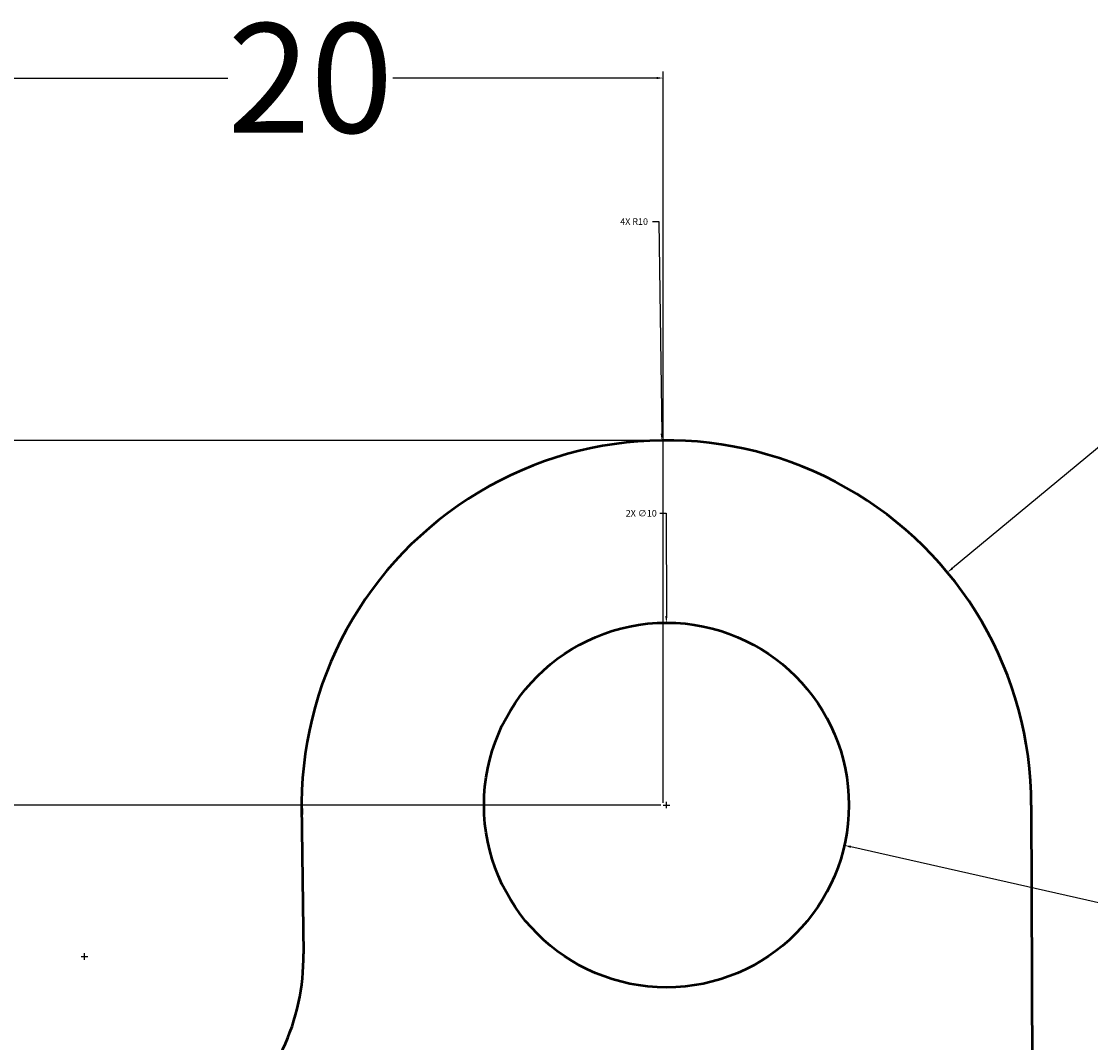
# Model space of a CAD drawing. Units: millimetres. Extents: x -53 to 92, y -147 to 37.
# Tile 15 of 16: x 11 to 40, y 9 to 37. Entities that reach past the tile are written whole.
import ezdxf

# ---------------------------------------------------------------- set-up
doc = ezdxf.new("R2010")
doc.units = ezdxf.units.MM
doc.header["$MEASUREMENT"] = 0
doc.layers.add('M-DIMS', color=2, linetype='Continuous', lineweight=25)
doc.layers.add('M-OUTL', color=7, linetype='Continuous', lineweight=50)
doc.styles.get("Standard").update_dxf_attribs({"font": 'arial.ttf'})
doc.dimstyles.get("Standard").update_dxf_attribs({"dimtxt": 0.18, "dimasz": 0.18, "dimexe": 0.18, "dimexo": 0.0625, "dimgap": 0.09, "dimtad": 0, "dimtih": 1, "dimtoh": 1, "dimdec": 4, "dimzin": 0, "dimdsep": 46, "dimtxsty": 'Standard', "dimcen": 0.09, "dimadec": 0, "dimazin": 0, "dimtfac": 1, "dimtdec": 4, "dimtofl": 0, "dimtmove": 0, "dimatfit": 3, "dimfxl": 1, "dimtolj": 1, "dimtzin": 0, "dimarcsym": 0})

# ---------------------------------------------------------------- blocks, each defined once
blk = doc.blocks.new('*D1')
at = {"layer": 'Defpoints', "color": 0, "transparency": 16777216}
for p in [(36.393, 22.289), (28.692, 15.91)]:
    blk.add_point(p, dxfattribs=at)
at = {"layer": 'M-DIMS', "color": 0, "lineweight": -2, "transparency": 16777216}
for p, q in [((52.762, 35.845), (36.532, 22.403)), ((52.942, 35.845), (52.762, 35.845)), ((28.602, 15.91), (28.782, 15.91)), ((28.692, 15.82), (28.692, 16))]:
    blk.add_line(p, q, dxfattribs=at)
at = {"layer": 'M-DIMS', "color": 0, "transparency": 16777216}
blk.add_solid([(36.513, 22.426), (36.551, 22.38), (36.393, 22.289)], dxfattribs=at)
at = {"layer": 'M-DIMS', "color": 0, "transparency": 16777216, "insert": (56.611, 35.845), "char_height": 0.18, "attachment_point": 5}
blk.add_mtext('\\A1;{\\H16.66667x;R10}', dxfattribs=at)
blk = doc.blocks.new('*D3')
at = {"layer": 'Defpoints', "color": 0, "transparency": 16777216}
for p in [(23.816, 17.015), (33.568, 14.805)]:
    blk.add_point(p, dxfattribs=at)
at = {"layer": 'M-DIMS', "color": 0, "lineweight": -2, "transparency": 16777216}
for p, q in [((28.602, 15.91), (28.782, 15.91)), ((28.692, 15.82), (28.692, 16)), ((47.959, 11.542), (33.744, 14.765))]:
    blk.add_line(p, q, dxfattribs=at)
at = {"layer": 'M-DIMS', "color": 0, "transparency": 16777216}
blk.add_solid([(33.75, 14.794), (33.737, 14.736), (33.568, 14.805)], dxfattribs=at)
at = {"layer": 'M-DIMS', "color": 0, "transparency": 16777216, "insert": (51.824, 11.542), "char_height": 0.18, "attachment_point": 5}
blk.add_mtext('\\A1;{\\H16.66667x;%%C10}', dxfattribs=at)
blk = doc.blocks.new('*D5')
at = {"layer": 'Defpoints', "color": 0, "transparency": 16777216}
for p in [(28.602, 35.845), (28.602, 15.91), (9.265, -3.88)]:
    blk.add_point(p, dxfattribs=at)
at = {"layer": 'M-DIMS', "color": 0, "lineweight": -2, "transparency": 16777216}
for p, q in [((9.265, -3.817), (9.265, 36.025)), ((9.445, 35.845), (16.674, 35.845)), ((28.422, 35.845), (21.192, 35.845)), ((28.602, 15.973), (28.602, 36.025))]:
    blk.add_line(p, q, dxfattribs=at)
at = {"layer": 'M-DIMS', "color": 0, "transparency": 16777216}
for points in [[(9.445, 35.875), (9.445, 35.815), (9.265, 35.845)], [(28.422, 35.875), (28.422, 35.815), (28.602, 35.845)]]:
    blk.add_solid(points, dxfattribs=at)
at = {"layer": 'M-DIMS', "color": 0, "transparency": 16777216, "insert": (18.933, 35.845), "char_height": 0.18, "attachment_point": 5}
blk.add_mtext('\\A1;{\\H16.66667x;20}', dxfattribs=at)
blk = doc.blocks.new('*D6')
at = {"layer": 'Defpoints', "color": 0, "transparency": 16777216}
for p in [(-26.95, 15.91), (28.602, 15.91), (9.355, -3.79)]:
    blk.add_point(p, dxfattribs=at)
at = {"layer": 'M-DIMS', "color": 0, "lineweight": -2, "transparency": 16777216}
for p, q in [((28.539, 15.91), (-27.13, 15.91)), ((-26.95, 15.73), (-26.95, 7.682)), ((-26.95, -3.61), (-26.95, 4.438)), ((9.292, -3.79), (-27.13, -3.79))]:
    blk.add_line(p, q, dxfattribs=at)
at = {"layer": 'M-DIMS', "color": 0, "transparency": 16777216}
for points in [[(-26.98, 15.73), (-26.92, 15.73), (-26.95, 15.91)], [(-26.98, -3.61), (-26.92, -3.61), (-26.95, -3.79)]]:
    blk.add_solid(points, dxfattribs=at)
at = {"layer": 'M-DIMS', "color": 0, "transparency": 16777216, "insert": (-26.95, 6.06), "char_height": 0.18, "attachment_point": 5}
blk.add_mtext('\\A1;{\\H16.66667x;20}', dxfattribs=at)
blk = doc.blocks.new('HOLE-D10')
blk.add_circle((5, 5), 5)
blk = doc.blocks.new('*D17')
at = {"layer": 'Defpoints', "color": 0, "transparency": 16777216}
for p in [(-46.81, 25.909), (28.564, 25.909), (18.165, -111.975)]:
    blk.add_point(p, dxfattribs=at)
at = {"layer": 'M-DIMS', "color": 0, "lineweight": -2, "transparency": 16777216}
for p, q in [((28.502, 25.909), (-46.99, 25.909)), ((-46.81, 25.729), (-46.81, -42.851)), ((-46.81, -111.795), (-46.81, -43.215)), ((18.102, -111.975), (-46.99, -111.975))]:
    blk.add_line(p, q, dxfattribs=at)
at = {"layer": 'M-DIMS', "color": 0, "transparency": 16777216}
for points in [[(-46.84, 25.729), (-46.78, 25.729), (-46.81, 25.909)], [(-46.84, -111.795), (-46.78, -111.795), (-46.81, -111.975)]]:
    blk.add_solid(points, dxfattribs=at)
at = {"layer": 'M-DIMS', "color": 0, "transparency": 16777216, "insert": (-46.81, -43.033), "char_height": 0.18, "attachment_point": 5}
blk.add_mtext('\\A1;137.88', dxfattribs=at)
blk = doc.blocks.new('*D19')
at = {"layer": 'Defpoints', "color": 0, "transparency": 16777216}
for p in [(28.69, 20.91), (28.694, 10.91)]:
    blk.add_point(p, dxfattribs=at)
at = {"layer": 'M-DIMS', "color": 0, "lineweight": -2, "transparency": 16777216}
for p, q in [((28.509, 23.91), (28.689, 23.91)), ((28.689, 23.91), (28.69, 21.09)), ((28.602, 15.91), (28.782, 15.91)), ((28.692, 15.82), (28.692, 16))]:
    blk.add_line(p, q, dxfattribs=at)
at = {"layer": 'M-DIMS', "color": 0, "transparency": 16777216}
blk.add_solid([(28.72, 21.09), (28.66, 21.09), (28.69, 20.91)], dxfattribs=at)
at = {"layer": 'M-DIMS', "color": 0, "transparency": 16777216, "insert": (28.002, 23.91), "char_height": 0.18, "attachment_point": 5}
blk.add_mtext('\\A1;2X ∅10', dxfattribs=at)
blk = doc.blocks.new('*D20')
at = {"layer": 'Defpoints', "color": 0, "transparency": 16777216}
for p in [(28.564, 25.909), (28.692, 15.91)]:
    blk.add_point(p, dxfattribs=at)
at = {"layer": 'M-DIMS', "color": 0, "lineweight": -2, "transparency": 16777216}
for p, q in [((28.307, 31.909), (28.487, 31.909)), ((28.487, 31.909), (28.562, 26.089)), ((28.602, 15.91), (28.782, 15.91)), ((28.692, 15.82), (28.692, 16))]:
    blk.add_line(p, q, dxfattribs=at)
at = {"layer": 'M-DIMS', "color": 0, "transparency": 16777216}
blk.add_solid([(28.592, 26.09), (28.532, 26.089), (28.564, 25.909)], dxfattribs=at)
at = {"layer": 'M-DIMS', "color": 0, "transparency": 16777216, "insert": (27.806, 31.909), "char_height": 0.18, "attachment_point": 5}
blk.add_mtext('\\A1;4X R10', dxfattribs=at)
blk = doc.blocks.new('*D21')
at = {"layer": 'Defpoints', "color": 0, "transparency": 16777216}
for p in [(12.745, 11.757), (16.541, 7.111)]:
    blk.add_point(p, dxfattribs=at)
at = {"layer": 'M-DIMS', "color": 0, "lineweight": -2, "transparency": 16777216}
for p, q in [((12.655, 11.757), (12.835, 11.757)), ((12.745, 11.667), (12.745, 11.847)), ((18.819, 4.323), (16.655, 6.971)), ((18.999, 4.323), (18.819, 4.323))]:
    blk.add_line(p, q, dxfattribs=at)
at = {"layer": 'M-DIMS', "color": 0, "transparency": 16777216}
blk.add_solid([(16.678, 6.99), (16.632, 6.953), (16.541, 7.111)], dxfattribs=at)
at = {"layer": 'M-DIMS', "color": 0, "transparency": 16777216, "insert": (19.427, 4.323), "char_height": 0.18, "attachment_point": 5}
blk.add_mtext('\\A1;3X R6', dxfattribs=at)

msp = doc.modelspace()

# ---------------------------------------------------------------- linework, layer by layer
at = {"layer": 'M-OUTL'}
for p, q in [((18.69189, 15.91719), (18.74409, 11.83368)), ((38.69188, 15.90293), (38.97226, -58.39443))]:
    msp.add_line(p, q, dxfattribs=at)
for centre, radius, start, end in [((28.69189, 15.91006), 10, 359.959148, 181.505579), ((12.74458, 11.75699), 6, 257.767876, 0.732363)]:
    msp.add_arc(centre, radius, start, end, dxfattribs=at)

# ---------------------------------------------------------------- block references
msp.add_blockref('HOLE-D10', (23.692, 10.91), dxfattribs=at)

# ---------------------------------------------------------------- dimensions: what is measured, and where the dimension line sits
at = {"layer": 'M-DIMS'}
dim = msp.add_linear_dim(base=(28.60189, 35.84496), p1=(9.26461, -3.87977), p2=(28.60189, 15.91006), text='{\\H16.66667x;20}', dimstyle='Standard', override={"dimclrd": 0, "dimclre": 0, "dimclrt": 0}, dxfattribs=at)
dim.commit()
dim.dimension.update_dxf_attribs({"geometry": '*D5', "text_midpoint": (18.93325, 35.84496)})
for center, mpoint, text, override, picture, middle in [((28.69189, 15.91006), (36.39347, 22.28858), '{\\H16.66667x;R10}', {"dimclrd": 0, "dimclre": 0, "dimclrt": 0}, '*D1', (56.61093, 35.84496)), ((28.69189, 15.91006), (28.564, 25.90924), '4X <>', {"dimdec": 0, "dimlfac": 1, "dimrnd": 0, "dimzin": 0, "dimdsep": 46, "dimlunit": 2}, '*D20', (27.80551, 31.90875)), ((12.74458, 11.75699), (16.5411, 7.11087), '3X <>', {"dimdec": 0, "dimlfac": 1, "dimrnd": 0, "dimzin": 0, "dimdsep": 46, "dimlunit": 2}, '*D21', (19.42741, 4.3232))]:
    dim = msp.add_radius_dim(center=center, mpoint=mpoint, text=text, dimstyle='Standard', override=override, dxfattribs=at)
    dim.commit()
    dim.dimension.update_dxf_attribs({"geometry": picture, "text_midpoint": middle, "dimtype": 164})
dim = msp.add_linear_dim(base=(-46.8103, 25.90924), p1=(18.16452, -111.97467), p2=(28.56407, 25.90924), angle=90, dimstyle='Standard', override={"dimdec": 2, "dimlfac": 1, "dimrnd": 0, "dimzin": 0, "dimdsep": 46, "dimlunit": 2}, dxfattribs=at)
dim.commit()
dim.dimension.update_dxf_attribs({"geometry": '*D17', "text_midpoint": (-46.8103, -43.03271)})
for p1, p2, text, override, picture, middle in [((28.69377, 10.91006), (28.69, 20.91005), '2X <>', {"dimdec": 0, "dimlfac": 1, "dimrnd": 0, "dimzin": 0, "dimdsep": 46, "dimlunit": 2}, '*D19', (28.0022, 23.91005)), ((23.81561, 17.01547), (33.56816, 14.80464), '{\\H16.66667x;%%C10}', {"dimclrd": 0, "dimclre": 0, "dimclrt": 0}, '*D3', (47.95869, 11.54241))]:
    dim = msp.add_diameter_dim_2p(p1=p1, p2=p2, text=text, dimstyle='Standard', override=override, dxfattribs=at)
    dim.commit()
    dim.dimension.update_dxf_attribs({"geometry": picture, "text_midpoint": middle, "dimtype": 163})
dim = msp.add_linear_dim(base=(-26.95014, 15.91006), p1=(9.35461, -3.78977), p2=(28.60189, 15.91006), angle=90, text='{\\H16.66667x;20}', dimstyle='Standard', override={"dimclrd": 0, "dimclre": 0, "dimclrt": 0}, dxfattribs=at)
dim.commit()
dim.dimension.update_dxf_attribs({"geometry": '*D6', "text_midpoint": (-26.95014, 6.06014)})

doc.saveas('drawing.dxf')
